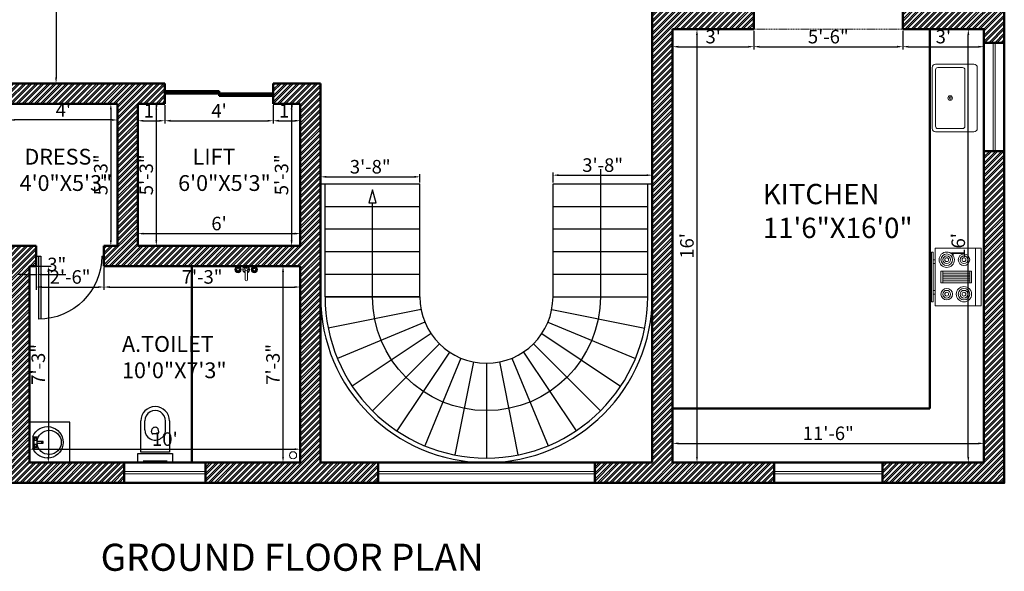
# Model space of a CAD drawing. Units: inches. Extents: x 3590 to 5167, y 65 to 1917.
# Tile 5 of 100: x 3869 to 4306, y 70 to 314. Entities that reach past the tile are written whole.
import ezdxf

# ---------------------------------------------------------------- set-up
doc = ezdxf.new("R2010")
doc.units = ezdxf.units.IN
doc.linetypes.add('DASHED', pattern=[0.75, 0.5, -0.25])
for name, color, linetype, lineweight in [('A-ANNO-DIMS', 2, 'Continuous', 18), ('A-ANNO-TEXT', 7, 'Continuous', 25), ('A-AREA-IDEN', 7, 'Continuous', 18), ('A-DOOR', 3, 'Continuous', 25), ('A-FLOR-FIXT', 8, 'Continuous', 18), ('A-FLOR-STRS', 7, 'Continuous', 25), ('A-GLAZ', 4, 'Continuous', 18), ('A-WALL', 7, 'Continuous', 50), ('A-WALL-PATT', 251, 'Continuous', 13), ('S-BEAM-OVHD', 7, 'DASHED', 18)]:
    doc.layers.add(name, color=color, linetype=linetype, lineweight=lineweight)
doc.layers.add('SANTEH', color=7, linetype='Continuous')
doc.styles.get("Standard").update_dxf_attribs({"font": 'arial.ttf'})
doc.dimstyles.new('ISO-25', dxfattribs={"dimtxt": 9, "dimasz": 2.5, "dimexe": 1.25, "dimexo": 0.625, "dimtad": 1, "dimdec": 1, "dimlunit": 3, "dimtxsty": 'Standard', "dimcen": 2.5, "dimadec": 0, "dimazin": 0, "dimtfac": 1, "dimtdec": 1, "dimtmove": 0, "dimatfit": 3, "dimfxl": 1, "dimarcsym": 0})

# ---------------------------------------------------------------- blocks, each defined once
blk = doc.blocks.new('*U160')
blk.add_line((-21, 0), (21, 0))
blk = doc.blocks.new('*U161')
at = {"layer": 'A-FLOR-STRS', "color": 0, "linetype": 'ByBlock', "lineweight": -2, "transparency": 16777216}
for p, rotation in [((4076.01, 1459), 89.99999999999982), ((4066.16, 1458.03), 101.2499999999998), ((4085.86, 1458.03), 78.7499999999998), ((4056.69, 1455.15), 112.4999999999998), ((4095.34, 1455.15), 67.4999999999998), ((4047.96, 1450.49), 123.7499999999997), ((4104.07, 1450.49), 56.24999999999984), ((4040.3, 1444.21), 134.9999999999996), ((4111.72, 1444.21), 44.99999999999992), ((4034.02, 1436.56), 146.2499999999996), ((4118, 1436.56), 33.74999999999991), ((4029.36, 1427.82), 157.4999999999995), ((4122.67, 1427.82), 22.49999999999996), ((4026.48, 1418.35), 168.7499999999995), ((4125.54, 1418.35), 11.25), ((4025.51, 1408.5), 180)]:
    blk.add_blockref('*U160', p, dxfattribs=dict(at, rotation=rotation))
blk.add_blockref('*U160', (4126.51, 1408.5), dxfattribs=at)
blk = doc.blocks.new('D2')
for p, q in [((1, 0), (1, 28)), ((2, 0), (2, 27.98)), ((0, 0), (2, 0)), ((29, 0), (30, 0))]:
    blk.add_line(p, q)
at = {"ltscale": 0.5}
blk.add_arc((1, 0), 28, 0, 90, dxfattribs=at)
blk = doc.blocks.new('*D173')
at = {"layer": 'A-ANNO-DIMS', "color": 0, "lineweight": -2, "transparency": 16777216}
for p, q in [((3864.51, 276.43), (3864.51, 268.61)), ((3912.51, 276.43), (3912.51, 268.61)), ((3910.01, 269.86), (3867.01, 269.86))]:
    blk.add_line(p, q, dxfattribs=at)
at = {"layer": 'A-ANNO-DIMS', "color": 0, "transparency": 16777216}
for points in [[(3867.01, 270.28), (3867.01, 269.44), (3864.51, 269.86)], [(3910.01, 270.28), (3910.01, 269.44), (3912.51, 269.86)]]:
    blk.add_solid(points, dxfattribs=at)
at = {"layer": 'Defpoints', "color": 0, "transparency": 16777216}
for p in [(3864.51, 277.06), (3912.51, 277.06), (3864.51, 269.86)]:
    blk.add_point(p, dxfattribs=at)
at = {"layer": 'A-ANNO-DIMS', "color": 0, "transparency": 16777216, "insert": (3888.51, 273.49), "char_height": 6, "attachment_point": 5}
blk.add_mtext("4'", dxfattribs=at)
blk = doc.blocks.new('*D174')
at = {"layer": 'A-ANNO-DIMS', "color": 0, "lineweight": -2, "transparency": 16777216}
for p, q in [((3911.89, 277.06), (3908.31, 277.06)), ((3909.56, 274.56), (3909.56, 216.56)), ((3911.89, 214.06), (3908.31, 214.06))]:
    blk.add_line(p, q, dxfattribs=at)
at = {"layer": 'A-ANNO-DIMS', "color": 0, "transparency": 16777216}
for points in [[(3909.14, 274.56), (3909.98, 274.56), (3909.56, 277.06)], [(3909.14, 216.56), (3909.98, 216.56), (3909.56, 214.06)]]:
    blk.add_solid(points, dxfattribs=at)
at = {"layer": 'Defpoints', "color": 0, "transparency": 16777216}
for p in [(3912.51, 277.06), (3909.56, 214.06), (3912.51, 214.06)]:
    blk.add_point(p, dxfattribs=at)
at = {"layer": 'A-ANNO-DIMS', "color": 0, "transparency": 16777216, "insert": (3905.87, 245.56), "char_height": 6, "attachment_point": 5, "rotation": 90}
blk.add_mtext('5\'-3"', dxfattribs=at)
blk = doc.blocks.new('*D175')
at = {"layer": 'A-ANNO-DIMS', "color": 0, "lineweight": -2, "transparency": 16777216}
for p, q in [((3871.01, 201.37), (3868.51, 201.37)), ((3873.51, 204.43), (3873.51, 200.12)), ((3873.51, 201.37), (3876.51, 201.37)), ((3876.51, 204.43), (3876.51, 200.12)), ((3879.01, 201.37), (3889.65, 201.37))]:
    blk.add_line(p, q, dxfattribs=at)
at = {"layer": 'A-ANNO-DIMS', "color": 0, "transparency": 16777216}
for points in [[(3871.01, 201.79), (3871.01, 200.95), (3873.51, 201.37)], [(3879.01, 201.79), (3879.01, 200.95), (3876.51, 201.37)]]:
    blk.add_solid(points, dxfattribs=at)
at = {"layer": 'Defpoints', "color": 0, "transparency": 16777216}
for p in [(3873.51, 205.06), (3876.51, 205.06), (3876.51, 201.37)]:
    blk.add_point(p, dxfattribs=at)
at = {"layer": 'A-ANNO-DIMS', "color": 0, "transparency": 16777216, "insert": (3885.58, 205.06), "char_height": 6, "attachment_point": 5}
blk.add_mtext('3"', dxfattribs=at)
blk = doc.blocks.new('*D213')
at = {"layer": 'A-ANNO-DIMS', "color": 0, "lineweight": -2, "transparency": 16777216}
for p, q in [((3876.51, 204.43), (3876.51, 194.58)), ((3906.51, 204.43), (3906.51, 194.58)), ((3879.01, 195.83), (3904.01, 195.83))]:
    blk.add_line(p, q, dxfattribs=at)
at = {"layer": 'A-ANNO-DIMS', "color": 0, "transparency": 16777216}
for points in [[(3879.01, 196.25), (3879.01, 195.42), (3876.51, 195.83)], [(3904.01, 196.25), (3904.01, 195.42), (3906.51, 195.83)]]:
    blk.add_solid(points, dxfattribs=at)
at = {"layer": 'Defpoints', "color": 0, "transparency": 16777216}
for p in [(3876.51, 205.06), (3906.51, 205.06), (3906.51, 195.83)]:
    blk.add_point(p, dxfattribs=at)
at = {"layer": 'A-ANNO-DIMS', "color": 0, "transparency": 16777216, "insert": (3891.51, 199.52), "char_height": 6, "attachment_point": 5}
blk.add_mtext('2\'-6"', dxfattribs=at)
blk = doc.blocks.new('*D214')
at = {"layer": 'A-ANNO-DIMS', "color": 0, "lineweight": -2, "transparency": 16777216}
for p, q in [((3906.51, 204.43), (3906.51, 194.58)), ((3993.51, 204.43), (3993.51, 194.58)), ((3909.01, 195.83), (3991.01, 195.83))]:
    blk.add_line(p, q, dxfattribs=at)
at = {"layer": 'A-ANNO-DIMS', "color": 0, "transparency": 16777216}
for points in [[(3909.01, 196.25), (3909.01, 195.42), (3906.51, 195.83)], [(3991.01, 196.25), (3991.01, 195.42), (3993.51, 195.83)]]:
    blk.add_solid(points, dxfattribs=at)
at = {"layer": 'Defpoints', "color": 0, "transparency": 16777216}
for p in [(3906.51, 205.06), (3993.51, 205.06), (3993.51, 195.83)]:
    blk.add_point(p, dxfattribs=at)
at = {"layer": 'A-ANNO-DIMS', "color": 0, "transparency": 16777216, "insert": (3950.01, 199.53), "char_height": 6, "attachment_point": 5}
blk.add_mtext('7\'-3"', dxfattribs=at)
blk = doc.blocks.new('*D215')
at = {"layer": 'A-ANNO-DIMS', "color": 0, "lineweight": -2, "transparency": 16777216}
for p, q in [((3874.14, 205.06), (3883.11, 205.06)), ((3881.86, 202.56), (3881.86, 120.56)), ((3874.14, 118.06), (3883.11, 118.06))]:
    blk.add_line(p, q, dxfattribs=at)
at = {"layer": 'A-ANNO-DIMS', "color": 0, "transparency": 16777216}
for points in [[(3881.44, 202.56), (3882.28, 202.56), (3881.86, 205.06)], [(3881.44, 120.56), (3882.28, 120.56), (3881.86, 118.06)]]:
    blk.add_solid(points, dxfattribs=at)
at = {"layer": 'Defpoints', "color": 0, "transparency": 16777216}
for p in [(3873.51, 205.06), (3873.51, 118.06), (3881.86, 118.06)]:
    blk.add_point(p, dxfattribs=at)
at = {"layer": 'A-ANNO-DIMS', "color": 0, "transparency": 16777216, "insert": (3878.17, 161.56), "char_height": 6, "attachment_point": 5, "rotation": 90}
blk.add_mtext('7\'-3"', dxfattribs=at)
blk = doc.blocks.new('*D216')
at = {"layer": 'A-ANNO-DIMS', "color": 0, "lineweight": -2, "transparency": 16777216}
for p, q in [((3873.51, 118.68), (3873.51, 125.22)), ((3876.01, 123.97), (3991.01, 123.97)), ((3993.51, 118.68), (3993.51, 125.22))]:
    blk.add_line(p, q, dxfattribs=at)
at = {"layer": 'A-ANNO-DIMS', "color": 0, "transparency": 16777216}
for points in [[(3876.01, 124.39), (3876.01, 123.56), (3873.51, 123.97)], [(3991.01, 124.39), (3991.01, 123.56), (3993.51, 123.97)]]:
    blk.add_solid(points, dxfattribs=at)
at = {"layer": 'Defpoints', "color": 0, "transparency": 16777216}
for p in [(3993.51, 123.97), (3873.51, 118.06), (3993.51, 118.06)]:
    blk.add_point(p, dxfattribs=at)
at = {"layer": 'A-ANNO-DIMS', "color": 0, "transparency": 16777216, "insert": (3933.51, 127.66), "char_height": 6, "attachment_point": 5}
blk.add_mtext("10'", dxfattribs=at)
blk = doc.blocks.new('*D181')
at = {"layer": 'A-ANNO-DIMS', "color": 0, "lineweight": -2, "transparency": 16777216}
for p, q in [((3992.89, 205.06), (3984.62, 205.06)), ((3985.87, 120.56), (3985.87, 202.56)), ((3992.89, 118.06), (3984.62, 118.06))]:
    blk.add_line(p, q, dxfattribs=at)
at = {"layer": 'A-ANNO-DIMS', "color": 0, "transparency": 16777216}
for points in [[(3985.45, 202.56), (3986.29, 202.56), (3985.87, 205.06)], [(3985.45, 120.56), (3986.29, 120.56), (3985.87, 118.06)]]:
    blk.add_solid(points, dxfattribs=at)
at = {"layer": 'Defpoints', "color": 0, "transparency": 16777216}
for p in [(3985.87, 205.06), (3993.51, 205.06), (3993.51, 118.06)]:
    blk.add_point(p, dxfattribs=at)
at = {"layer": 'A-ANNO-DIMS', "color": 0, "transparency": 16777216, "insert": (3982.18, 161.56), "char_height": 6, "attachment_point": 5, "rotation": 90}
blk.add_mtext('7\'-3"', dxfattribs=at)
blk = doc.blocks.new('*D182')
at = {"layer": 'A-ANNO-DIMS', "color": 0, "lineweight": -2, "transparency": 16777216}
for p, q in [((3921.51, 214.68), (3921.51, 220.75)), ((3924.01, 219.5), (3991.01, 219.5)), ((3993.51, 214.68), (3993.51, 220.75))]:
    blk.add_line(p, q, dxfattribs=at)
at = {"layer": 'A-ANNO-DIMS', "color": 0, "transparency": 16777216}
for points in [[(3924.01, 219.92), (3924.01, 219.08), (3921.51, 219.5)], [(3991.01, 219.92), (3991.01, 219.08), (3993.51, 219.5)]]:
    blk.add_solid(points, dxfattribs=at)
at = {"layer": 'Defpoints', "color": 0, "transparency": 16777216}
for p in [(3993.51, 219.5), (3921.51, 214.06), (3993.51, 214.06)]:
    blk.add_point(p, dxfattribs=at)
at = {"layer": 'A-ANNO-DIMS', "color": 0, "transparency": 16777216, "insert": (3957.51, 223.19), "char_height": 6, "attachment_point": 5}
blk.add_mtext("6'", dxfattribs=at)
blk = doc.blocks.new('*D183')
at = {"layer": 'A-ANNO-DIMS', "color": 0, "lineweight": -2, "transparency": 16777216}
for p, q in [((3922.14, 277.06), (3930.95, 277.06)), ((3929.7, 274.56), (3929.7, 216.56)), ((3922.14, 214.06), (3930.95, 214.06))]:
    blk.add_line(p, q, dxfattribs=at)
at = {"layer": 'A-ANNO-DIMS', "color": 0, "transparency": 16777216}
for points in [[(3929.29, 274.56), (3930.12, 274.56), (3929.7, 277.06)], [(3929.29, 216.56), (3930.12, 216.56), (3929.7, 214.06)]]:
    blk.add_solid(points, dxfattribs=at)
at = {"layer": 'Defpoints', "color": 0, "transparency": 16777216}
for p in [(3921.51, 277.06), (3921.51, 214.06), (3929.7, 214.06)]:
    blk.add_point(p, dxfattribs=at)
at = {"layer": 'A-ANNO-DIMS', "color": 0, "transparency": 16777216, "insert": (3926.01, 245.56), "char_height": 6, "attachment_point": 5, "rotation": 90}
blk.add_mtext('5\'-3"', dxfattribs=at)
blk = doc.blocks.new('*D184')
at = {"layer": 'A-ANNO-DIMS', "color": 0, "lineweight": -2, "transparency": 16777216}
for p, q in [((3992.89, 277.06), (3988.42, 277.06)), ((3989.67, 274.56), (3989.67, 216.56)), ((3992.89, 214.06), (3988.42, 214.06))]:
    blk.add_line(p, q, dxfattribs=at)
at = {"layer": 'A-ANNO-DIMS', "color": 0, "transparency": 16777216}
for points in [[(3989.25, 274.56), (3990.09, 274.56), (3989.67, 277.06)], [(3989.25, 216.56), (3990.09, 216.56), (3989.67, 214.06)]]:
    blk.add_solid(points, dxfattribs=at)
at = {"layer": 'Defpoints', "color": 0, "transparency": 16777216}
for p in [(3993.51, 277.06), (3989.67, 214.06), (3993.51, 214.06)]:
    blk.add_point(p, dxfattribs=at)
at = {"layer": 'A-ANNO-DIMS', "color": 0, "transparency": 16777216, "insert": (3985.98, 245.56), "char_height": 6, "attachment_point": 5, "rotation": 90}
blk.add_mtext('5\'-3"', dxfattribs=at)
blk = doc.blocks.new('*D185')
at = {"layer": 'A-ANNO-DIMS', "color": 0, "lineweight": -2, "transparency": 16777216}
for p, q in [((3921.51, 276.43), (3921.51, 268.28)), ((3933.51, 276.43), (3933.51, 268.28)), ((3924.01, 269.53), (3931.01, 269.53))]:
    blk.add_line(p, q, dxfattribs=at)
at = {"layer": 'A-ANNO-DIMS', "color": 0, "transparency": 16777216}
for points in [[(3924.01, 269.94), (3924.01, 269.11), (3921.51, 269.53)], [(3931.01, 269.94), (3931.01, 269.11), (3933.51, 269.53)]]:
    blk.add_solid(points, dxfattribs=at)
at = {"layer": 'Defpoints', "color": 0, "transparency": 16777216}
for p in [(3921.51, 277.06), (3933.51, 277.06), (3933.51, 269.53)]:
    blk.add_point(p, dxfattribs=at)
at = {"layer": 'A-ANNO-DIMS', "color": 0, "transparency": 16777216, "insert": (3927.51, 273.16), "char_height": 6, "attachment_point": 5}
blk.add_mtext("1'", dxfattribs=at)
blk = doc.blocks.new('*D168')
at = {"layer": 'A-ANNO-DIMS', "color": 0, "lineweight": -2, "transparency": 16777216}
for p, q in [((3933.51, 276.43), (3933.51, 268.28)), ((3981.51, 276.43), (3981.51, 268.28)), ((3936.01, 269.53), (3979.01, 269.53))]:
    blk.add_line(p, q, dxfattribs=at)
at = {"layer": 'A-ANNO-DIMS', "color": 0, "transparency": 16777216}
for points in [[(3936.01, 269.94), (3936.01, 269.11), (3933.51, 269.53)], [(3979.01, 269.94), (3979.01, 269.11), (3981.51, 269.53)]]:
    blk.add_solid(points, dxfattribs=at)
at = {"layer": 'Defpoints', "color": 0, "transparency": 16777216}
for p in [(3933.51, 277.06), (3981.51, 277.06), (3981.51, 269.53)]:
    blk.add_point(p, dxfattribs=at)
at = {"layer": 'A-ANNO-DIMS', "color": 0, "transparency": 16777216, "insert": (3957.51, 273.15), "char_height": 6, "attachment_point": 5}
blk.add_mtext("4'", dxfattribs=at)
blk = doc.blocks.new('*D169')
at = {"layer": 'A-ANNO-DIMS', "color": 0, "lineweight": -2, "transparency": 16777216}
for p, q in [((3981.51, 276.43), (3981.51, 268.28)), ((3993.51, 276.43), (3993.51, 268.28)), ((3984.01, 269.53), (3991.01, 269.53))]:
    blk.add_line(p, q, dxfattribs=at)
at = {"layer": 'A-ANNO-DIMS', "color": 0, "transparency": 16777216}
for points in [[(3984.01, 269.94), (3984.01, 269.11), (3981.51, 269.53)], [(3991.01, 269.94), (3991.01, 269.11), (3993.51, 269.53)]]:
    blk.add_solid(points, dxfattribs=at)
at = {"layer": 'Defpoints', "color": 0, "transparency": 16777216}
for p in [(3981.51, 277.06), (3993.51, 277.06), (3993.51, 269.53)]:
    blk.add_point(p, dxfattribs=at)
at = {"layer": 'A-ANNO-DIMS', "color": 0, "transparency": 16777216, "insert": (3987.51, 273.16), "char_height": 6, "attachment_point": 5}
blk.add_mtext("1'", dxfattribs=at)
blk = doc.blocks.new('*D170')
at = {"layer": 'A-ANNO-DIMS', "color": 0, "lineweight": -2, "transparency": 16777216}
for p, q in [((4158.51, 118.68), (4158.51, 127.79)), ((4296.51, 118.68), (4296.51, 127.79)), ((4161.01, 126.54), (4294.01, 126.54))]:
    blk.add_line(p, q, dxfattribs=at)
at = {"layer": 'A-ANNO-DIMS', "color": 0, "transparency": 16777216}
for points in [[(4161.01, 126.95), (4161.01, 126.12), (4158.51, 126.54)], [(4294.01, 126.95), (4294.01, 126.12), (4296.51, 126.54)]]:
    blk.add_solid(points, dxfattribs=at)
at = {"layer": 'Defpoints', "color": 0, "transparency": 16777216}
for p in [(4296.51, 126.54), (4158.51, 118.06), (4296.51, 118.06)]:
    blk.add_point(p, dxfattribs=at)
at = {"layer": 'A-ANNO-DIMS', "color": 0, "transparency": 16777216, "insert": (4227.51, 130.23), "char_height": 6, "attachment_point": 5}
blk.add_mtext('11\'-6"', dxfattribs=at)
blk = doc.blocks.new('*D171')
at = {"layer": 'A-ANNO-DIMS', "color": 0, "lineweight": -2, "transparency": 16777216}
for p, q in [((4159.14, 310.06), (4170.56, 310.06)), ((4169.31, 307.56), (4169.31, 120.56)), ((4159.14, 118.06), (4170.56, 118.06))]:
    blk.add_line(p, q, dxfattribs=at)
at = {"layer": 'A-ANNO-DIMS', "color": 0, "transparency": 16777216}
for points in [[(4168.89, 307.56), (4169.72, 307.56), (4169.31, 310.06)], [(4168.89, 120.56), (4169.72, 120.56), (4169.31, 118.06)]]:
    blk.add_solid(points, dxfattribs=at)
at = {"layer": 'Defpoints', "color": 0, "transparency": 16777216}
for p in [(4158.51, 310.06), (4158.51, 118.06), (4169.31, 118.06)]:
    blk.add_point(p, dxfattribs=at)
at = {"layer": 'A-ANNO-DIMS', "color": 0, "transparency": 16777216, "insert": (4165.62, 214.06), "char_height": 6, "attachment_point": 5, "rotation": 90}
blk.add_mtext("16'", dxfattribs=at)
blk = doc.blocks.new('*D249')
at = {"layer": 'A-ANNO-DIMS', "color": 0, "lineweight": -2, "transparency": 16777216}
for p, q in [((4295.89, 310.06), (4288.31, 310.06)), ((4289.56, 120.56), (4289.56, 307.56)), ((4295.89, 118.06), (4288.31, 118.06))]:
    blk.add_line(p, q, dxfattribs=at)
at = {"layer": 'A-ANNO-DIMS', "color": 0, "transparency": 16777216}
for points in [[(4289.15, 307.56), (4289.98, 307.56), (4289.56, 310.06)], [(4289.15, 120.56), (4289.98, 120.56), (4289.56, 118.06)]]:
    blk.add_solid(points, dxfattribs=at)
at = {"layer": 'Defpoints', "color": 0, "transparency": 16777216}
for p in [(4289.56, 310.06), (4296.51, 310.06), (4296.51, 118.06)]:
    blk.add_point(p, dxfattribs=at)
at = {"layer": 'A-ANNO-DIMS', "color": 0, "transparency": 16777216, "insert": (4285.88, 214.06), "char_height": 6, "attachment_point": 5, "rotation": 90}
blk.add_mtext("16'", dxfattribs=at)
blk = doc.blocks.new('*D250')
at = {"layer": 'A-ANNO-DIMS', "color": 0, "lineweight": -2, "transparency": 16777216}
for p, q in [((4158.51, 309.43), (4158.51, 301.08)), ((4194.51, 309.43), (4194.51, 301.08)), ((4161.01, 302.33), (4192.01, 302.33))]:
    blk.add_line(p, q, dxfattribs=at)
at = {"layer": 'A-ANNO-DIMS', "color": 0, "transparency": 16777216}
for points in [[(4161.01, 302.75), (4161.01, 301.92), (4158.51, 302.33)], [(4192.01, 302.75), (4192.01, 301.92), (4194.51, 302.33)]]:
    blk.add_solid(points, dxfattribs=at)
at = {"layer": 'Defpoints', "color": 0, "transparency": 16777216}
for p in [(4158.51, 310.06), (4194.51, 310.06), (4194.51, 302.33)]:
    blk.add_point(p, dxfattribs=at)
at = {"layer": 'A-ANNO-DIMS', "color": 0, "transparency": 16777216, "insert": (4176.51, 306.02), "char_height": 6, "attachment_point": 5}
blk.add_mtext("3'", dxfattribs=at)
blk = doc.blocks.new('*D251')
at = {"layer": 'A-ANNO-DIMS', "color": 0, "lineweight": -2, "transparency": 16777216}
for p, q in [((4194.51, 309.43), (4194.51, 301.08)), ((4260.51, 309.43), (4260.51, 301.08)), ((4197.01, 302.33), (4258.01, 302.33))]:
    blk.add_line(p, q, dxfattribs=at)
at = {"layer": 'A-ANNO-DIMS', "color": 0, "transparency": 16777216}
for points in [[(4197.01, 302.75), (4197.01, 301.92), (4194.51, 302.33)], [(4258.01, 302.75), (4258.01, 301.92), (4260.51, 302.33)]]:
    blk.add_solid(points, dxfattribs=at)
at = {"layer": 'Defpoints', "color": 0, "transparency": 16777216}
for p in [(4194.51, 310.06), (4260.51, 310.06), (4260.51, 302.33)]:
    blk.add_point(p, dxfattribs=at)
at = {"layer": 'A-ANNO-DIMS', "color": 0, "transparency": 16777216, "insert": (4227.51, 306.02), "char_height": 6, "attachment_point": 5}
blk.add_mtext('5\'-6"', dxfattribs=at)
blk = doc.blocks.new('*D252')
at = {"layer": 'A-ANNO-DIMS', "color": 0, "lineweight": -2, "transparency": 16777216}
for p, q in [((4260.51, 309.43), (4260.51, 301.08)), ((4296.51, 309.43), (4296.51, 301.08)), ((4263.01, 302.33), (4294.01, 302.33))]:
    blk.add_line(p, q, dxfattribs=at)
at = {"layer": 'A-ANNO-DIMS', "color": 0, "transparency": 16777216}
for points in [[(4263.01, 302.75), (4263.01, 301.92), (4260.51, 302.33)], [(4294.01, 302.75), (4294.01, 301.92), (4296.51, 302.33)]]:
    blk.add_solid(points, dxfattribs=at)
at = {"layer": 'Defpoints', "color": 0, "transparency": 16777216}
for p in [(4260.51, 310.06), (4296.51, 310.06), (4296.51, 302.33)]:
    blk.add_point(p, dxfattribs=at)
at = {"layer": 'A-ANNO-DIMS', "color": 0, "transparency": 16777216, "insert": (4278.51, 306.02), "char_height": 6, "attachment_point": 5}
blk.add_mtext("3'", dxfattribs=at)
blk = doc.blocks.new('*D188')
at = {"layer": 'A-ANNO-DIMS', "color": 0, "lineweight": -2, "transparency": 16777216}
for p, q in [((3874.14, 580.06), (3886.54, 580.06)), ((3885.29, 577.56), (3885.29, 288.56)), ((3874.14, 286.06), (3886.54, 286.06))]:
    blk.add_line(p, q, dxfattribs=at)
at = {"layer": 'A-ANNO-DIMS', "color": 0, "transparency": 16777216}
for points in [[(3884.87, 577.56), (3885.7, 577.56), (3885.29, 580.06)], [(3884.87, 288.56), (3885.7, 288.56), (3885.29, 286.06)]]:
    blk.add_solid(points, dxfattribs=at)
at = {"layer": 'Defpoints', "color": 0, "transparency": 16777216}
for p in [(3873.51, 580.06), (3873.51, 286.06), (3885.29, 286.06)]:
    blk.add_point(p, dxfattribs=at)
at = {"layer": 'A-ANNO-DIMS', "color": 0, "transparency": 16777216, "insert": (3881.6, 433.06), "char_height": 6, "attachment_point": 5, "rotation": 90}
blk.add_mtext('24\'-6"', dxfattribs=at)
blk = doc.blocks.new('Range-Oven - 30 in top')
for p, q in [((0, -3), (30, -3)), ((12, -6), (18, -6)), ((13, -20), (13, -6)), ((14, -6), (14, -20)), ((15, -20), (15, -6)), ((16, -6), (16, -20)), ((17, -20), (17, -6)), ((18, -20), (12, -20)), ((6, -24), (6, -25)), ((8, -25), (8, -24)), ((22, -25), (22, -24)), ((24, -24), (24, -25))]:
    blk.add_line(p, q)
for points in [[(0, -24), (0, 0), (30, 0), (30, -24)], [(12, -21), (12, -5), (18, -5), (18, -21)], [(2, -26), (2, -25), (28, -25), (28, -26)]]:
    blk.add_lwpolyline(points, close=True)
for centre, radius in [((6, -9), 4), ((6, -9), 3), ((6, -9), 2), ((6, -9), 1), ((24, -9), 3), ((24, -9), 2), ((24, -9), 1), ((6, -18), 3), ((24, -18), 4), ((24, -18), 3), ((6, -18), 2), ((6, -18), 1), ((24, -18), 2), ((24, -18), 1)]:
    blk.add_circle(centre, radius)
blk = doc.blocks.new('Sink-single - 30 in top')
blk.add_line((-15, -3.999996), (15, -3.999996))
for points in [[(-13.5, 0), (13.5, 0)], [(-15, -18.499996), (-15, -1.5)], [(15, -1.5), (15, -18.499996)], [(-13.5, -17.499996), (-13.5, -6.499996)], [(-12.5, -5.499996), (12.5, -5.499996)], [(13.5, -6.499996), (13.5, -17.499996)], [(13.5, -19.999996), (-13.5, -19.999996)], [(12.5, -18.499996), (-12.5, -18.499996)]]:
    blk.add_lwpolyline(points)
for radius in [1, 0.5]:
    blk.add_circle((0, -11.999996), radius)
for centre, radius, start, end in [((-13.5, -1.5), 1.5, 90, 180), ((13.5, -1.5), 1.5, 0, 90), ((-12.5, -6.499996), 1, 90, 180), ((12.5, -6.499996), 1, 0, 90), ((-13.5, -18.499996), 1.5, 180, 270), ((-12.5, -17.499996), 1, 180, 270), ((12.5, -17.499996), 1, 270, 0), ((13.5, -18.499996), 1.5, 270, 0)]:
    blk.add_arc(centre, radius, start, end)
blk = doc.blocks.new('y3')
at = {"layer": 'SANTEH', "ltscale": 5}
for p, q in [((38, 131), (38, 521)), ((88, 411), (88, 521)), ((347, 426), (348, 521)), ((398, 521), (398, 131)), ((172, 385), (181, 421)), ((263, 385), (254, 421)), ((244, 358), (191, 358)), ((398, 131), (38, 131)), ((67, 21), (367, 21))]:
    blk.add_line(p, q, dxfattribs=at)
blk.add_lwpolyline([(0, 115), (435, 115), (435, 0), (0, 0), (0, 115)], dxfattribs=at)
for centre, radius, start, end in [((218, 521), 180, 0, 180), ((218, 521), 130, 359.1579, 180), ((218, 411), 130, 180, 5.9855), ((191, 378), 20, 160.5038, 270), ((218, 400), 42.2, 30.5234, 149.4766), ((244, 378), 20, 270, 19.4962)]:
    blk.add_arc(centre, radius, start, end, dxfattribs=at)
blk = doc.blocks.new('r11')
at = {"layer": 'SANTEH', "ltscale": 5}
for p, q in [((0, 0), (600, 0)), ((0, -600), (0, 0)), ((600, 0), (600, -600)), ((210, -50), (390, -50)), ((210, -50), (210, -50)), ((224, -63), (376, -63)), ((224, -113), (224, -63)), ((376, -113), (224, -113)), ((233, -79), (249, -69)), ((233, -98), (233, -79)), ((249, -107), (233, -98)), ((249, -69), (266, -79)), ((266, -98), (249, -107)), ((266, -79), (266, -98)), ((288, -202), (288, -113)), ((312, -113), (312, -202)), ((334, -79), (351, -69)), ((334, -98), (334, -79)), ((351, -107), (334, -98)), ((351, -69), (367, -79)), ((367, -98), (351, -107)), ((367, -79), (367, -98)), ((376, -63), (376, -113)), ((312, -184), (288, -184)), ((312, -202), (288, -202)), ((600, -600), (0, -600))]:
    blk.add_line(p, q, dxfattribs=at)
for centre, radius, start, end in [((300, -266), 234, 112.5, 67.5), ((300, -293), 180, 93.8183, 86.1817)]:
    blk.add_arc(centre, radius, start, end, dxfattribs=at)
blk = doc.blocks.new('Faucet - Bathroom top')
for p, q in [((-4.107, 0.125), (-4.375, 0.125)), ((-3.75, 0.4788), (-3.75, 0.75)), ((-3.5, 0.482), (-3.5, 0.75)), ((-3.1461, 0.125), (-2.875, 0.125)), ((3.143, 0.125), (2.875, 0.125)), ((3.5, 0.4788), (3.5, 0.75)), ((3.75, 0.482), (3.75, 0.75)), ((4.1039, 0.125), (4.375, 0.125)), ((-4.1039, -0.125), (-4.375, -0.125)), ((-3.75, -0.4821), (-3.75, -0.75)), ((-3.5, -0.4789), (-3.5, -0.75)), ((-3.143, -0.125), (-2.875, -0.125)), ((-0.5, -0.8639), (-0.5, -4.5)), ((0.5, -4.5), (0.5, -0.8631)), ((3.1461, -0.125), (2.875, -0.125)), ((3.5, -0.4821), (3.5, -0.75)), ((3.75, -0.4789), (3.75, -0.75)), ((4.107, -0.125), (4.375, -0.125))]:
    blk.add_line(p, q)
for centre, radius in [((-3.625, 0), 1.375), ((-4.625, 0), 0.2795), ((-3.625, 0), 0.5), ((-3.625, 1), 0.2795), ((-2.625, 0), 0.2795), ((0, 0), 0.5), ((3.625, 0), 1.375), ((2.625, 0), 0.2795), ((3.625, 0), 0.5), ((3.625, 1), 0.2795), ((4.625, 0), 0.2795), ((-3.625, -1), 0.2795), ((3.625, -1), 0.2795)]:
    blk.add_circle(centre, radius)
for centre, radius, start, end in [((-3.625, 0), 1, 105.2407, 164.2093), ((-3.625, 0), 1, 16.44125, 74.07887), ((0, 0), 1.5, 289.6514, 250.3603), ((0, 0), 1, 300.3431, 239.7554), ((3.625, 0), 1, 106.12, 164.0884), ((3.625, 0), 1, 16.23422, 73.90469), ((-3.625, 0), 1, 196.2342, 253.9047), ((-3.625, 0), 1, 286.12, 344.0884), ((3.625, 0), 1, 196.4413, 254.0789), ((3.625, 0), 1, 285.2407, 344.2093), ((0, -4.5), 0.5, 180, 0)]:
    blk.add_arc(centre, radius, start, end)
blk = doc.blocks.new('*D283')
at = {"layer": 'A-ANNO-DIMS', "color": 0, "lineweight": -2, "transparency": 16777216}
for p, q in [((4002.51, 242.18), (4002.51, 245.92)), ((4005.01, 244.67), (4044.01, 244.67)), ((4046.51, 242.18), (4046.51, 245.92))]:
    blk.add_line(p, q, dxfattribs=at)
at = {"layer": 'A-ANNO-DIMS', "color": 0, "transparency": 16777216}
for points in [[(4005.01, 245.08), (4005.01, 244.25), (4002.51, 244.67)], [(4044.01, 245.08), (4044.01, 244.25), (4046.51, 244.67)]]:
    blk.add_solid(points, dxfattribs=at)
at = {"layer": 'Defpoints', "color": 0, "transparency": 16777216}
for p in [(4046.51, 244.67), (4002.51, 241.56), (4046.51, 241.56)]:
    blk.add_point(p, dxfattribs=at)
at = {"layer": 'A-ANNO-DIMS', "color": 0, "transparency": 16777216, "insert": (4024.51, 248.36), "char_height": 6, "attachment_point": 5}
blk.add_mtext('3\'-8"', dxfattribs=at)
blk = doc.blocks.new('*D284')
at = {"layer": 'A-ANNO-DIMS', "color": 0, "lineweight": -2, "transparency": 16777216}
for p, q in [((4105.51, 242.18), (4105.51, 246.65)), ((4108.01, 245.4), (4147.01, 245.4)), ((4149.51, 242.18), (4149.51, 246.65))]:
    blk.add_line(p, q, dxfattribs=at)
at = {"layer": 'A-ANNO-DIMS', "color": 0, "transparency": 16777216}
for points in [[(4108.01, 245.81), (4108.01, 244.98), (4105.51, 245.4)], [(4147.01, 245.81), (4147.01, 244.98), (4149.51, 245.4)]]:
    blk.add_solid(points, dxfattribs=at)
at = {"layer": 'Defpoints', "color": 0, "transparency": 16777216}
for p in [(4149.51, 245.4), (4105.51, 241.56), (4149.51, 241.56)]:
    blk.add_point(p, dxfattribs=at)
at = {"layer": 'A-ANNO-DIMS', "color": 0, "transparency": 16777216, "insert": (4127.51, 249.09), "char_height": 6, "attachment_point": 5}
blk.add_mtext('3\'-8"', dxfattribs=at)

msp = doc.modelspace()

# ---------------------------------------------------------------- hatches: boundary and pattern name
at = {"layer": 'A-WALL-PATT', "transparency": 33554687}
h = msp.add_hatch(dxfattribs=at)
h.set_pattern_fill('ANSI32', color=256, scale=0.2)
h.set_pattern_definition([(45, (0, -1216.9392), (-1.3470384, 1.3470384), []), (45, (0.898, -1216.9392), (-1.3470384, 1.3470384), [])])
h.paths.add_polyline_path([(3768.51, 589.06), (3645.51, 589.06), (3645.51, 568.06), (3654.51, 568.06), (3654.51, 580.06), (3671.16, 580.06), (3768.51, 580.06)])
h.paths.add_polyline_path([(3909.51, 589.06), (3816.51, 589.06), (3816.51, 580.06), (3864.51, 580.06), (3864.51, 574.06), (3873.51, 574.06), (3873.51, 580.06), (3909.51, 580.06)])
h.paths.add_polyline_path([(4053.51, 589.06), (3969.51, 589.06), (3969.51, 580.06), (4053.51, 580.06)])
h.paths.add_polyline_path([(4215.51, 589.06), (4113.51, 589.06), (4113.51, 580.06), (4206.51, 580.06), (4206.51, 574.06), (4215.51, 574.06)])
h.paths.add_polyline_path([(3654.51, 520.06), (3645.51, 520.06), (3645.51, 403.06), (3654.51, 403.06), (3654.51, 433.06), (3741.51, 433.06), (3741.51, 439.06), (3654.51, 439.06)], flags=17)
h.paths.add_polyline_path([(3873.51, 538.06), (3864.51, 538.06), (3864.51, 439.06), (3771.51, 439.06), (3771.51, 433.06), (3774.51, 433.06), (3774.51, 337.06), (3654.51, 337.06), (3654.51, 367.06), (3645.51, 367.06), (3645.51, 322.06), (3654.51, 322.06), (3654.51, 328.06), (3864.51, 328.06), (3864.51, 322.06), (3873.51, 322.06), (3873.51, 367.06), (3864.51, 367.06), (3864.51, 337.06), (3780.51, 337.06), (3780.51, 433.06), (3864.51, 433.06), (3864.51, 403.06), (3873.51, 403.06)])
h.paths.add_polyline_path([(3654.51, 274.06), (3645.51, 274.06), (3645.51, 109.06), (3810.51, 109.06), (3810.51, 118.06), (3809.96, 118.06), (3654.51, 118.06)])
h.paths.add_polyline_path([(3915.51, 118.06), (3873.51, 118.06), (3873.51, 135.93), (3873.51, 205.06), (3876.51, 205.06), (3876.51, 214.06), (3864.51, 214.06), (3864.51, 118.06), (3858.51, 118.06), (3858.51, 109.06), (3915.51, 109.06)])
h.paths.add_polyline_path([(4028.01, 118.06), (4002.51, 118.06), (4002.51, 286.06), (3981.51, 286.06), (3981.51, 277.06), (3993.51, 277.06), (3993.51, 214.06), (3921.51, 214.06), (3921.51, 277.06), (3933.51, 277.06), (3933.51, 286.06), (3864.51, 286.06), (3864.51, 277.06), (3912.51, 277.06), (3912.51, 214.06), (3906.51, 214.06), (3906.51, 205.06), (3993.51, 205.06), (3993.51, 118.06), (3951.51, 118.06), (3951.51, 109.06), (4028.01, 109.06)])
h.paths.add_polyline_path([(4203.51, 118.06), (4158.51, 118.06), (4158.51, 310.06), (4194.51, 310.06), (4194.51, 319.06), (4149.51, 319.06), (4149.51, 118.06), (4124.01, 118.06), (4124.01, 109.06), (4203.51, 109.06)])
h.paths.add_polyline_path([(4305.51, 349.06), (4296.51, 349.06), (4296.51, 319.06), (4278.64, 319.06), (4260.51, 319.06), (4260.51, 310.06), (4296.51, 310.06), (4296.51, 304.06), (4305.51, 304.06)])
h.paths.add_polyline_path([(4305.51, 256.06), (4296.51, 256.06), (4296.51, 118.06), (4251.51, 118.06), (4251.51, 109.06), (4305.51, 109.06)])
h.paths.add_polyline_path([(4305.51, 460.06), (4215.51, 460.06), (4215.51, 526.06), (4206.51, 526.06), (4206.51, 460.06), (4149.51, 460.06), (4149.51, 451.06), (4296.51, 451.06), (4296.51, 421.06), (4305.51, 421.06)])

# ---------------------------------------------------------------- linework, layer by layer
at = {"layer": 'A-FLOR-FIXT'}
msp.add_circle((3990.31, 121.27), 1.6, dxfattribs=at)
at = {"layer": 'A-FLOR-STRS'}
for p, q in [((4002.51, 241.56), (4046.51, 241.56)), ((4004.51, 191.56), (4004.51, 241.56)), ((4046.51, 191.56), (4046.51, 241.56)), ((4105.51, 241.56), (4149.51, 241.56)), ((4105.51, 191.56), (4105.51, 241.56)), ((4147.51, 191.56), (4147.51, 241.56)), ((4004.51, 231.56), (4046.51, 231.56)), ((4105.51, 231.56), (4147.51, 231.56)), ((4004.51, 221.56), (4046.51, 221.56)), ((4105.51, 221.56), (4147.51, 221.56)), ((4004.51, 211.56), (4046.51, 211.56)), ((4105.51, 211.56), (4147.51, 211.56)), ((4004.51, 201.56), (4046.51, 201.56)), ((4105.51, 201.56), (4147.51, 201.56)), ((4004.51, 191.56), (4046.51, 191.56))]:
    msp.add_line(p, q, dxfattribs=at)
msp.add_lwpolyline([(4126.51, 248), (4126.51, 191.56, -1), (4025.51, 191.56), (4025.51, 233.17)], format="xyb", dxfattribs=at)
msp.add_lwpolyline([(4025.51, 238.93), (4023.88, 233.17), (4027.15, 233.17)], close=True, dxfattribs=at)
for radius in [73.5, 71.5, 29.5]:
    msp.add_arc((4076.01, 191.56), radius, 180, 0, dxfattribs=at)
at = {"layer": 'A-GLAZ'}
for p, q in [((4300.51, 256.06), (4300.51, 304.06)), ((4301.51, 256.06), (4301.51, 304.06)), ((3951.51, 114.06), (3915.51, 114.06)), ((4124.01, 114.06), (4028.01, 114.06)), ((4251.51, 114.06), (4203.51, 114.06)), ((3951.51, 113.06), (3915.51, 113.06)), ((4124.01, 113.06), (4028.01, 113.06)), ((4251.51, 113.06), (4203.51, 113.06))]:
    msp.add_line(p, q, dxfattribs=at)
at = {"layer": 'A-WALL'}
for p, q in [((4149.51, 118.06), (4149.51, 319.06)), ((4194.51, 310.06), (4194.51, 319.06)), ((4260.51, 310.06), (4260.51, 319.06)), ((4194.51, 310.06), (4158.51, 310.06)), ((4158.51, 118.06), (4158.51, 310.06)), ((4296.51, 310.06), (4260.51, 310.06)), ((4272.51, 310.06), (4272.51, 142.06)), ((4296.51, 310.06), (4296.51, 118.06)), ((4305.51, 304.06), (4296.51, 304.06)), ((3933.51, 286.06), (3864.51, 286.06)), ((3933.51, 277.06), (3933.51, 286.06)), ((4002.51, 286.06), (3981.51, 286.06)), ((3981.51, 277.06), (3981.51, 286.06)), ((4002.51, 118.06), (4002.51, 286.06)), ((3933.51, 282.56), (3957.51, 282.56)), ((3933.51, 281.56), (3981.51, 281.56)), ((3957.51, 282.56), (3957.51, 280.56)), ((3957.51, 280.56), (3981.51, 280.56)), ((3912.51, 277.06), (3864.51, 277.06)), ((3912.51, 214.06), (3912.51, 277.06)), ((3933.51, 277.06), (3921.51, 277.06)), ((3921.51, 214.06), (3921.51, 277.06)), ((3993.51, 277.06), (3981.51, 277.06)), ((3993.51, 214.06), (3993.51, 277.06)), ((4305.51, 256.06), (4296.51, 256.06)), ((3876.51, 214.06), (3864.51, 214.06)), ((3876.51, 205.06), (3876.51, 214.06)), ((3912.51, 214.06), (3906.51, 214.06)), ((3906.51, 205.06), (3906.51, 214.06)), ((3993.51, 214.06), (3921.51, 214.06)), ((3876.51, 205.06), (3873.51, 205.06)), ((3873.51, 118.06), (3873.51, 205.06)), ((3993.51, 205.06), (3906.51, 205.06)), ((3945.51, 118.06), (3945.51, 205.06)), ((3993.51, 118.06), (3993.51, 205.06)), ((4272.51, 142.06), (4158.51, 142.06)), ((3993.51, 118.06), (3873.51, 118.06)), ((3915.51, 118.06), (3915.51, 109.06)), ((3951.51, 118.06), (3951.51, 109.06)), ((4149.51, 118.06), (4002.51, 118.06)), ((4028.01, 118.06), (4028.01, 109.06)), ((4124.01, 118.06), (4124.01, 109.06)), ((4296.51, 118.06), (4158.51, 118.06)), ((4203.51, 118.06), (4203.51, 109.06)), ((4251.51, 118.06), (4251.51, 109.06))]:
    msp.add_line(p, q, dxfattribs=at)
msp.add_lwpolyline([(4305.51, 460.06), (4305.51, 109.06), (3645.51, 109.06), (3645.51, 589.06), (4215.51, 589.06)], dxfattribs=at)
at = {"layer": 'S-BEAM-OVHD'}
msp.add_line((4194.51, 310.06), (4260.51, 310.06), dxfattribs=at)

# ---------------------------------------------------------------- block references
at = {"layer": 'A-DOOR', "xscale": -1, "rotation": 180}
msp.add_blockref('D2', (3876.51, 209.56), dxfattribs=at)
at = {"layer": 'A-FLOR-FIXT', "rotation": 270}
msp.add_blockref('Sink-single - 30 in top', (4293.53, 279.57), dxfattribs=at)
at = {"layer": 'A-FLOR-FIXT'}
for name, p, xscale, yscale, zscale, rotation in [('Range-Oven - 30 in top', (4295.27, 187.57), -0.8485281468519549, 0.8485281468519549, 0.8485281468519549, 270), ('r11', (3873.51, 135.93), -0.0297800069284724, 0.0297800069284724, 0.0297800069284724, 90)]:
    msp.add_blockref(name, p, dxfattribs=dict(at, xscale=xscale, yscale=yscale, zscale=zscale, rotation=rotation))
msp.add_blockref('Faucet - Bathroom top', (3969.55, 203.56), dxfattribs=at)
at = {"layer": 'A-FLOR-FIXT', "xscale": 0.0353848906415677, "yscale": 0.0353848906415677, "zscale": 0.0353848906415677}
msp.add_blockref('y3', (3921.48, 118.06), dxfattribs=at)
at = {"layer": 'A-FLOR-STRS', "xscale": -1, "rotation": 180}
msp.add_blockref('*U161', (0, 1600.06), dxfattribs=at)

# ---------------------------------------------------------------- texts
at = {"layer": 'A-ANNO-TEXT', "insert": (3905.03, 82.07), "char_height": 12, "attachment_point": 1}
msp.add_mtext_dynamic_manual_height_columns('{\\fTimes New Roman|b0|i0|c0|p18;GROUND FLOOR PLAN}', width=197.6934, gutter_width=12.5, heights=[0], dxfattribs=at)
at = {"layer": 'A-AREA-IDEN', "attachment_point": 1}
for s, insert, char_height in [('{\\fTimes New Roman|b0|i0|c0|p18; DRESS\\P4\'0"X5\'3"}', (3869.13, 257.09), 7), ('{\\fTimes New Roman|b0|i0|c0|p18;   LIFT\\P6\'0"X5\'3"}', (3939.39, 257.09), 7), ('{\\fTimes New Roman|b0|i0|c0|p18;KITCHEN\\P11\'6"X16\'0"}', (4198.48, 241.54), 9), ('{\\fTimes New Roman|b0|i0|c0|p18;A.TOILET\\P10\'0"X7\'3"}', (3914.52, 174.1), 7)]:
    msp.add_mtext_dynamic_manual_height_columns(s, width=67.3508, gutter_width=12.5, heights=[0], dxfattribs=dict(at, insert=insert, char_height=char_height))

# ---------------------------------------------------------------- dimensions: what is measured, and where the dimension line sits
at = {"layer": 'A-ANNO-DIMS'}
for base, p1, p2, picture, middle in [((3885.29, 286.06), (3873.51, 580.06), (3873.51, 286.06), '*D188', (3881.6, 433.06)), ((4169.31, 118.06), (4158.51, 310.06), (4158.51, 118.06), '*D171', (4165.62, 214.06)), ((4289.56, 310.06), (4296.51, 118.06), (4296.51, 310.06), '*D249', (4285.88, 214.06)), ((3909.56, 214.06), (3912.51, 277.06), (3912.51, 214.06), '*D174', (3905.87, 245.56)), ((3929.7, 214.06), (3921.51, 277.06), (3921.51, 214.06), '*D183', (3926.01, 245.56)), ((3989.67, 214.06), (3993.51, 277.06), (3993.51, 214.06), '*D184', (3985.98, 245.56)), ((3881.86, 118.06), (3873.51, 205.06), (3873.51, 118.06), '*D215', (3878.17, 161.56)), ((3985.87, 205.06), (3993.51, 118.06), (3993.51, 205.06), '*D181', (3982.18, 161.56))]:
    dim = msp.add_linear_dim(base=base, p1=p1, p2=p2, angle=90, dimstyle='ISO-25', override={"dimtxt": 6, "dimclrd": 0, "dimclre": 0, "dimclrt": 0}, dxfattribs=at)
    dim.commit()
    dim.dimension.update_dxf_attribs({"geometry": picture, "text_midpoint": middle})
for base, p1, p2, override, picture, middle in [((4194.51, 302.33), (4158.51, 310.06), (4194.51, 310.06), {"dimtxt": 6, "dimclrd": 0, "dimclre": 0, "dimclrt": 0}, '*D250', (4176.51, 306.02)), ((4260.51, 302.33), (4194.51, 310.06), (4260.51, 310.06), {"dimtxt": 6, "dimclrd": 0, "dimclre": 0, "dimclrt": 0, "dimtmove": 1}, '*D251', (4227.51, 306.02)), ((4296.51, 302.33), (4260.51, 310.06), (4296.51, 310.06), {"dimtxt": 6, "dimclrd": 0, "dimclre": 0, "dimclrt": 0, "dimtmove": 1}, '*D252', (4278.51, 306.02)), ((3864.51, 269.86), (3912.51, 277.06), (3864.51, 277.06), {"dimtxt": 6, "dimclrd": 0, "dimclre": 0, "dimclrt": 0}, '*D173', (3888.51, 273.49)), ((3933.51, 269.53), (3921.51, 277.06), (3933.51, 277.06), {"dimtxt": 6, "dimclrd": 0, "dimclre": 0, "dimclrt": 0}, '*D185', (3927.51, 273.16)), ((3981.51, 269.53), (3933.51, 277.06), (3981.51, 277.06), {"dimtxt": 6, "dimclrd": 0, "dimclre": 0, "dimclrt": 0, "dimtmove": 1}, '*D168', (3957.51, 273.15)), ((3993.51, 269.53), (3981.51, 277.06), (3993.51, 277.06), {"dimtxt": 6, "dimclrd": 0, "dimclre": 0, "dimclrt": 0, "dimtmove": 1}, '*D169', (3987.51, 273.16)), ((4149.51, 245.4), (4105.51, 241.56), (4149.51, 241.56), {"dimtxt": 6, "dimclrd": 0, "dimclre": 0, "dimclrt": 0}, '*D284', (4127.51, 249.09)), ((4046.51, 244.67), (4002.51, 241.56), (4046.51, 241.56), {"dimtxt": 6, "dimclrd": 0, "dimclre": 0, "dimclrt": 0}, '*D283', (4024.51, 248.36)), ((3993.51, 219.5), (3921.51, 214.06), (3993.51, 214.06), {"dimtxt": 6, "dimclrd": 0, "dimclre": 0, "dimclrt": 0}, '*D182', (3957.51, 223.19)), ((3876.51, 201.37), (3873.51, 205.06), (3876.51, 205.06), {"dimtxt": 6, "dimclrd": 0, "dimclre": 0, "dimclrt": 0}, '*D175', (3885.58, 205.06)), ((3906.51, 195.83), (3876.51, 205.06), (3906.51, 205.06), {"dimtxt": 6, "dimclrd": 0, "dimclre": 0, "dimclrt": 0, "dimtmove": 1}, '*D213', (3891.51, 199.52)), ((3993.51, 195.83), (3906.51, 205.06), (3993.51, 205.06), {"dimtxt": 6, "dimclrd": 0, "dimclre": 0, "dimclrt": 0, "dimtmove": 1}, '*D214', (3950.01, 199.53)), ((3993.51, 123.97), (3873.51, 118.06), (3993.51, 118.06), {"dimtxt": 6, "dimclrd": 0, "dimclre": 0, "dimclrt": 0}, '*D216', (3933.51, 127.66)), ((4296.51, 126.54), (4158.51, 118.06), (4296.51, 118.06), {"dimtxt": 6, "dimclrd": 0, "dimclre": 0, "dimclrt": 0}, '*D170', (4227.51, 130.23))]:
    dim = msp.add_linear_dim(base=base, p1=p1, p2=p2, dimstyle='ISO-25', override=override, dxfattribs=at)
    dim.commit()
    dim.dimension.update_dxf_attribs({"geometry": picture, "text_midpoint": middle})

doc.saveas('drawing.dxf')
